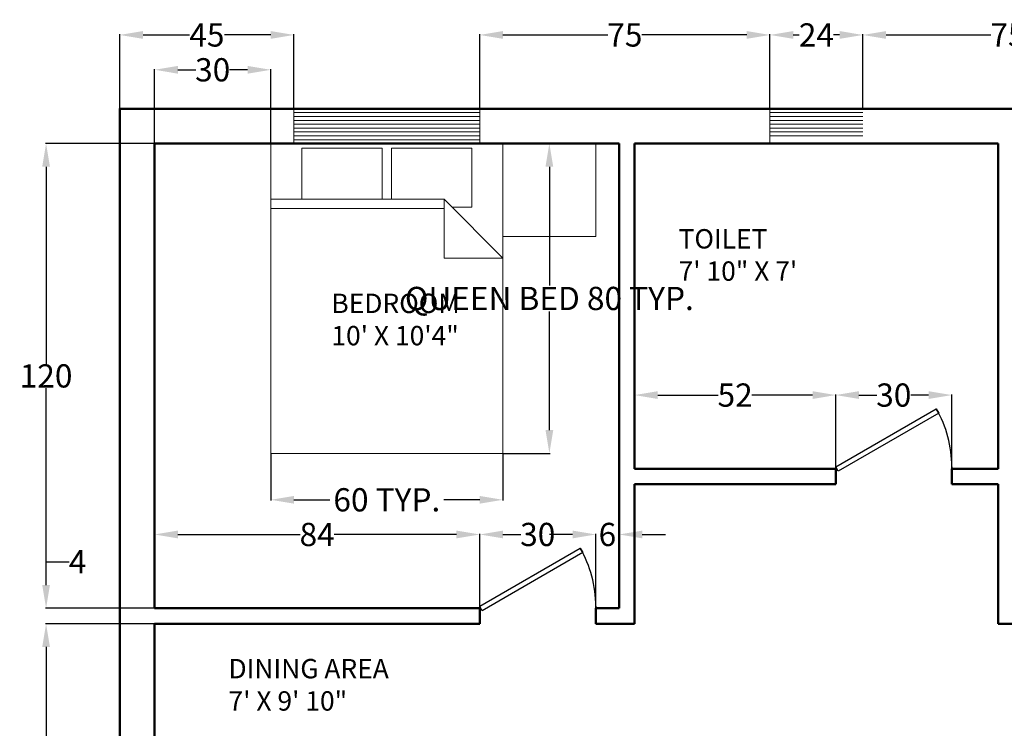
# Model space of a CAD drawing. Units: inches. Extents: x -8 to 445, y -363 to 43.
# Tile 2 of 3: x -8 to 246, y -140 to 43. Entities that reach past the tile are written whole.
import ezdxf

# ---------------------------------------------------------------- set-up
doc = ezdxf.new("R2010")
doc.units = ezdxf.units.IN
doc.header["$MEASUREMENT"] = 0
for name, color, linetype, lineweight in [('A-ANNO-DIMS', 2, 'Continuous', 18), ('A-AREA-IDEN', 7, 'Continuous', 18), ('A-FURN', 8, 'Continuous', 18), ('A-WALL', 7, 'Continuous', 50), ('DOORS', 43, 'Continuous', 25), ('WINDOWS', 140, 'Continuous', 18)]:
    doc.layers.add(name, color=color, linetype=linetype, lineweight=lineweight)
doc.styles.get("Standard").update_dxf_attribs({"font": 'arial.ttf'})
doc.dimstyles.get("Standard").update_dxf_attribs({"dimtxt": 6, "dimasz": 6, "dimexe": 0.18, "dimexo": 0.0625, "dimgap": 0.09, "dimtad": 0, "dimtih": 1, "dimtoh": 1, "dimdec": 0, "dimzin": 0, "dimdsep": 46, "dimlunit": 4, "dimtxsty": 'Standard', "dimcen": 0.09, "dimadec": 0, "dimazin": 0, "dimtfac": 1, "dimtdec": 0, "dimtofl": 0, "dimtmove": 0, "dimatfit": 3, "dimfxl": 1, "dimtolj": 1, "dimtzin": 0, "dimarcsym": 0})

# ---------------------------------------------------------------- blocks, each defined once
blk = doc.blocks.new('*U2')
for p, q in [((0, 0), (0, -6)), ((40, 0), (40, -6))]:
    blk.add_line(p, q)
blk.add_lwpolyline([(0, 0), (34.64, 20), (35.52, 18.48), (0.87, -1.52)], close=True)
blk.add_arc((0, 0), 40, 0, 30)
blk = doc.blocks.new('Bed - Queen')
for p, q in [((0, -80.00003), (0, 0)), ((0, 0), (59.99999, 0)), ((59.99999, 0), (59.99999, -80.00003)), ((7.99999, -1.2), (28.79998, -1.2)), ((7.99999, -14.4), (7.99999, -1.2)), ((28.79998, -1.2), (28.79998, -14.4)), ((31.19999, -1.2), (51.99999, -1.2)), ((31.19999, -14.4), (31.19999, -1.2)), ((51.99999, -1.2), (51.99999, -16.4)), ((0, -14.4), (44.8, -14.4)), ((59.99999, -29.6), (44.8, -14.4)), ((44.8, -14.4), (44.8, -29.6)), ((44.8, -16.8), (0, -16.8)), ((51.99999, -16.4), (46.79936, -16.4)), ((44.8, -29.6), (59.99999, -29.6)), ((59.99999, -80.00003), (0, -80.00003))]:
    blk.add_line(p, q)
blk = doc.blocks.new('WIN-48IN')
for p, q in [((0, 0), (0, 9)), ((0, 9), (48, 9)), ((0, 8), (48, 8)), ((48, 9), (48, 0)), ((0, 7), (48, 7)), ((0, 6), (48, 6)), ((0, 5), (48, 5)), ((0, 4), (48, 4)), ((0, 3), (48, 3)), ((0, 2), (48, 2)), ((48, 1), (0, 1)), ((48, 0), (0, 0))]:
    blk.add_line(p, q)
blk = doc.blocks.new('NIGHTSTAND-24IN')
blk.add_lwpolyline([(0, 24), (24, 24), (24, 0), (0, 0)], close=True)
blk = doc.blocks.new('*D17')
at = {"layer": 'A-ANNO-DIMS', "color": 0, "lineweight": -2, "transparency": 16777216}
for p, q in [((116.95, 10.91), (129.07, 10.91)), ((128.89, 4.91), (128.89, -25.71)), ((128.89, -63.09), (128.89, -32.47)), ((116.95, -69.09), (129.07, -69.09))]:
    blk.add_line(p, q, dxfattribs=at)
at = {"layer": 'A-ANNO-DIMS', "color": 0, "transparency": 16777216}
for points in [[(127.89, 4.91), (129.89, 4.91), (128.89, 10.91)], [(127.89, -63.09), (129.89, -63.09), (128.89, -69.09)]]:
    blk.add_solid(points, dxfattribs=at)
at = {"layer": 'Defpoints', "color": 0, "transparency": 16777216}
for p in [(116.89, 10.91), (128.89, 10.91), (116.89, -69.09)]:
    blk.add_point(p, dxfattribs=at)
at = {"layer": 'A-ANNO-DIMS', "color": 0, "transparency": 16777216, "insert": (128.89, -29.09), "char_height": 6, "attachment_point": 5}
blk.add_mtext('\\A1;QUEEN BED 80 TYP.', dxfattribs=at)
blk = doc.blocks.new('*D18')
at = {"layer": 'A-ANNO-DIMS', "color": 0, "lineweight": -2, "transparency": 16777216}
for p, q in [((56.89, -69.15), (56.89, -81.27)), ((116.89, -69.15), (116.89, -81.27)), ((62.89, -81.09), (72.18, -81.09)), ((110.89, -81.09), (101.6, -81.09))]:
    blk.add_line(p, q, dxfattribs=at)
at = {"layer": 'A-ANNO-DIMS', "color": 0, "transparency": 16777216}
for points in [[(62.89, -80.09), (62.89, -82.09), (56.89, -81.09)], [(110.89, -80.09), (110.89, -82.09), (116.89, -81.09)]]:
    blk.add_solid(points, dxfattribs=at)
at = {"layer": 'Defpoints', "color": 0, "transparency": 16777216}
for p in [(56.89, -69.09), (116.89, -69.09), (116.89, -81.09)]:
    blk.add_point(p, dxfattribs=at)
at = {"layer": 'A-ANNO-DIMS', "color": 0, "transparency": 16777216, "insert": (86.89, -81.09), "char_height": 6, "attachment_point": 5}
blk.add_mtext('\\A1;60 TYP.', dxfattribs=at)
blk = doc.blocks.new('*D35')
at = {"layer": 'A-ANNO-DIMS', "color": 0, "lineweight": -2, "transparency": 16777216}
for p, q in [((17.89, 19.97), (17.89, 39.14)), ((23.89, 38.96), (35.86, 38.96)), ((56.89, 38.96), (44.92, 38.96)), ((62.89, 19.97), (62.89, 39.14))]:
    blk.add_line(p, q, dxfattribs=at)
at = {"layer": 'A-ANNO-DIMS', "color": 0, "transparency": 16777216}
for points in [[(23.89, 39.96), (23.89, 37.96), (17.89, 38.96)], [(56.89, 39.96), (56.89, 37.96), (62.89, 38.96)]]:
    blk.add_solid(points, dxfattribs=at)
at = {"layer": 'Defpoints', "color": 0, "transparency": 16777216}
for p in [(62.89, 38.96), (17.89, 19.91), (62.89, 19.91)]:
    blk.add_point(p, dxfattribs=at)
at = {"layer": 'A-ANNO-DIMS', "color": 0, "transparency": 16777216, "insert": (40.39, 38.96), "char_height": 6, "attachment_point": 5}
blk.add_mtext('\\A1;45', dxfattribs=at)
blk = doc.blocks.new('*D36')
at = {"layer": 'A-ANNO-DIMS', "color": 0, "lineweight": -2, "transparency": 16777216}
for p, q in [((110.89, 19.97), (110.89, 39.14)), ((116.89, 38.96), (144, 38.96)), ((179.89, 38.96), (152.77, 38.96)), ((185.89, 19.97), (185.89, 39.14))]:
    blk.add_line(p, q, dxfattribs=at)
at = {"layer": 'A-ANNO-DIMS', "color": 0, "transparency": 16777216}
for points in [[(116.89, 39.96), (116.89, 37.96), (110.89, 38.96)], [(179.89, 39.96), (179.89, 37.96), (185.89, 38.96)]]:
    blk.add_solid(points, dxfattribs=at)
at = {"layer": 'Defpoints', "color": 0, "transparency": 16777216}
for p in [(185.89, 38.96), (110.89, 19.91), (185.89, 19.91)]:
    blk.add_point(p, dxfattribs=at)
at = {"layer": 'A-ANNO-DIMS', "color": 0, "transparency": 16777216, "insert": (148.39, 38.96), "char_height": 6, "attachment_point": 5}
blk.add_mtext('\\A1;75', dxfattribs=at)
blk = doc.blocks.new('*D37')
at = {"layer": 'A-ANNO-DIMS', "color": 0, "lineweight": -2, "transparency": 16777216}
for p, q in [((185.89, 19.97), (185.89, 39.14)), ((191.89, 38.96), (193.46, 38.96)), ((203.89, 38.96), (202.31, 38.96)), ((209.89, 19.97), (209.89, 39.14))]:
    blk.add_line(p, q, dxfattribs=at)
at = {"layer": 'A-ANNO-DIMS', "color": 0, "transparency": 16777216}
for points in [[(191.89, 39.96), (191.89, 37.96), (185.89, 38.96)], [(203.89, 39.96), (203.89, 37.96), (209.89, 38.96)]]:
    blk.add_solid(points, dxfattribs=at)
at = {"layer": 'Defpoints', "color": 0, "transparency": 16777216}
for p in [(209.89, 38.96), (185.89, 19.91), (209.89, 19.91)]:
    blk.add_point(p, dxfattribs=at)
at = {"layer": 'A-ANNO-DIMS', "color": 0, "transparency": 16777216, "insert": (197.89, 38.96), "char_height": 6, "attachment_point": 5}
blk.add_mtext('\\A1;24', dxfattribs=at)
blk = doc.blocks.new('*D38')
at = {"layer": 'A-ANNO-DIMS', "color": 0, "lineweight": -2, "transparency": 16777216}
for p, q in [((209.89, 19.97), (209.89, 39.14)), ((215.89, 38.96), (243, 38.96)), ((278.89, 38.96), (251.77, 38.96)), ((284.89, 19.97), (284.89, 39.14))]:
    blk.add_line(p, q, dxfattribs=at)
at = {"layer": 'A-ANNO-DIMS', "color": 0, "transparency": 16777216}
for points in [[(215.89, 39.96), (215.89, 37.96), (209.89, 38.96)], [(278.89, 39.96), (278.89, 37.96), (284.89, 38.96)]]:
    blk.add_solid(points, dxfattribs=at)
at = {"layer": 'Defpoints', "color": 0, "transparency": 16777216}
for p in [(284.89, 38.96), (209.89, 19.91), (284.89, 19.91)]:
    blk.add_point(p, dxfattribs=at)
at = {"layer": 'A-ANNO-DIMS', "color": 0, "transparency": 16777216, "insert": (247.39, 38.96), "char_height": 6, "attachment_point": 5}
blk.add_mtext('\\A1;75', dxfattribs=at)
blk = doc.blocks.new('*D39')
at = {"layer": 'A-ANNO-DIMS', "color": 0, "lineweight": -2, "transparency": 16777216}
for p, q in [((26.82, 10.91), (-1.34, 10.91)), ((-1.16, 4.91), (-1.16, -45.94)), ((-1.16, -103.09), (-1.16, -52.24)), ((26.82, -109.09), (-1.34, -109.09))]:
    blk.add_line(p, q, dxfattribs=at)
at = {"layer": 'A-ANNO-DIMS', "color": 0, "transparency": 16777216}
for points in [[(-2.16, 4.91), (-0.16, 4.91), (-1.16, 10.91)], [(-2.16, -103.09), (-0.16, -103.09), (-1.16, -109.09)]]:
    blk.add_solid(points, dxfattribs=at)
at = {"layer": 'Defpoints', "color": 0, "transparency": 16777216}
for p in [(-1.16, 10.91), (26.89, 10.91), (26.89, -109.09)]:
    blk.add_point(p, dxfattribs=at)
at = {"layer": 'A-ANNO-DIMS', "color": 0, "transparency": 16777216, "insert": (-1.16, -49.09), "char_height": 6, "attachment_point": 5}
blk.add_mtext('\\A1;120', dxfattribs=at)
blk = doc.blocks.new('*D40')
at = {"layer": 'A-ANNO-DIMS', "color": 0, "lineweight": -2, "transparency": 16777216}
for p, q in [((-1.16, -103.09), (-1.16, -97.09)), ((-1.16, -97.09), (4.84, -97.09)), ((26.82, -109.09), (-1.34, -109.09)), ((26.82, -113.09), (-1.34, -113.09)), ((-1.16, -119.09), (-1.16, -125.09))]:
    blk.add_line(p, q, dxfattribs=at)
at = {"layer": 'A-ANNO-DIMS', "color": 0, "transparency": 16777216}
for points in [[(-2.16, -103.09), (-0.16, -103.09), (-1.16, -109.09)], [(-2.16, -119.09), (-0.16, -119.09), (-1.16, -113.09)]]:
    blk.add_solid(points, dxfattribs=at)
at = {"layer": 'Defpoints', "color": 0, "transparency": 16777216}
for p in [(-1.16, -109.09), (26.89, -109.09), (26.89, -113.09)]:
    blk.add_point(p, dxfattribs=at)
at = {"layer": 'A-ANNO-DIMS', "color": 0, "transparency": 16777216, "insert": (7, -97.09), "char_height": 6, "attachment_point": 5}
blk.add_mtext('\\A1;4', dxfattribs=at)
blk = doc.blocks.new('*D41')
at = {"layer": 'A-ANNO-DIMS', "color": 0, "lineweight": -2, "transparency": 16777216}
for p, q in [((26.82, -113.09), (-1.34, -113.09)), ((-1.16, -119.09), (-1.16, -168.94)), ((-1.16, -225.09), (-1.16, -175.24)), ((26.82, -231.09), (-1.34, -231.09))]:
    blk.add_line(p, q, dxfattribs=at)
at = {"layer": 'A-ANNO-DIMS', "color": 0, "transparency": 16777216}
for points in [[(-2.16, -119.09), (-0.16, -119.09), (-1.16, -113.09)], [(-2.16, -225.09), (-0.16, -225.09), (-1.16, -231.09)]]:
    blk.add_solid(points, dxfattribs=at)
at = {"layer": 'Defpoints', "color": 0, "transparency": 16777216}
for p in [(-1.16, -113.09), (26.89, -113.09), (26.89, -231.09)]:
    blk.add_point(p, dxfattribs=at)
at = {"layer": 'A-ANNO-DIMS', "color": 0, "transparency": 16777216, "insert": (-1.16, -172.09), "char_height": 6, "attachment_point": 5}
blk.add_mtext('\\A1;118', dxfattribs=at)
blk = doc.blocks.new('*D50')
at = {"layer": 'A-ANNO-DIMS', "color": 0, "lineweight": -2, "transparency": 16777216}
for p, q in [((110.89, -109.03), (110.89, -89.86)), ((116.89, -90.04), (121.51, -90.04)), ((134.89, -90.04), (130.26, -90.04)), ((140.89, -109.03), (140.89, -89.86))]:
    blk.add_line(p, q, dxfattribs=at)
at = {"layer": 'A-ANNO-DIMS', "color": 0, "transparency": 16777216}
for points in [[(116.89, -89.04), (116.89, -91.04), (110.89, -90.04)], [(134.89, -89.04), (134.89, -91.04), (140.89, -90.04)]]:
    blk.add_solid(points, dxfattribs=at)
at = {"layer": 'Defpoints', "color": 0, "transparency": 16777216}
for p in [(140.89, -90.04), (110.89, -109.09), (140.89, -109.09)]:
    blk.add_point(p, dxfattribs=at)
at = {"layer": 'A-ANNO-DIMS', "color": 0, "transparency": 16777216, "insert": (125.89, -90.04), "char_height": 6, "attachment_point": 5}
blk.add_mtext('\\A1;30', dxfattribs=at)
blk = doc.blocks.new('*D51')
at = {"layer": 'A-ANNO-DIMS', "color": 0, "lineweight": -2, "transparency": 16777216}
for p, q in [((26.89, -109.03), (26.89, -89.86)), ((32.89, -90.04), (64.51, -90.04)), ((104.89, -90.04), (73.27, -90.04)), ((110.89, -109.03), (110.89, -89.86))]:
    blk.add_line(p, q, dxfattribs=at)
at = {"layer": 'A-ANNO-DIMS', "color": 0, "transparency": 16777216}
for points in [[(32.89, -89.04), (32.89, -91.04), (26.89, -90.04)], [(104.89, -89.04), (104.89, -91.04), (110.89, -90.04)]]:
    blk.add_solid(points, dxfattribs=at)
at = {"layer": 'Defpoints', "color": 0, "transparency": 16777216}
for p in [(110.89, -90.04), (26.89, -109.09), (110.89, -109.09)]:
    blk.add_point(p, dxfattribs=at)
at = {"layer": 'A-ANNO-DIMS', "color": 0, "transparency": 16777216, "insert": (68.89, -90.04), "char_height": 6, "attachment_point": 5}
blk.add_mtext('\\A1;84', dxfattribs=at)
blk = doc.blocks.new('*D52')
at = {"layer": 'A-ANNO-DIMS', "color": 0, "lineweight": -2, "transparency": 16777216}
for p, q in [((134.887242, -90.040687), (128.887242, -90.040687)), ((140.887242, -109.028187), (140.887242, -89.860687)), ((146.887242, -109.028187), (146.887242, -89.860687)), ((152.887242, -90.040687), (158.887242, -90.040687))]:
    blk.add_line(p, q, dxfattribs=at)
at = {"layer": 'A-ANNO-DIMS', "color": 0, "transparency": 16777216}
for points in [[(134.887242, -89.040687), (134.887242, -91.040687), (140.887242, -90.040687)], [(152.887242, -89.040687), (152.887242, -91.040687), (146.887242, -90.040687)]]:
    blk.add_solid(points, dxfattribs=at)
at = {"layer": 'Defpoints', "color": 0, "transparency": 16777216}
for p in [(146.887242, -90.040687), (140.887242, -109.090687), (146.887242, -109.090687)]:
    blk.add_point(p, dxfattribs=at)
at = {"layer": 'A-ANNO-DIMS', "color": 0, "transparency": 16777216, "insert": (143.887242, -90.040687), "char_height": 6, "attachment_point": 5}
blk.add_mtext('\\A1;6', dxfattribs=at)
blk = doc.blocks.new('*D53')
at = {"layer": 'A-ANNO-DIMS', "color": 0, "lineweight": -2, "transparency": 16777216}
for p, q in [((150.89, -73.03), (150.89, -53.86)), ((156.89, -54.04), (172.53, -54.04)), ((196.89, -54.04), (181.24, -54.04)), ((202.89, -73.03), (202.89, -53.86))]:
    blk.add_line(p, q, dxfattribs=at)
at = {"layer": 'A-ANNO-DIMS', "color": 0, "transparency": 16777216}
for points in [[(156.89, -53.04), (156.89, -55.04), (150.89, -54.04)], [(196.89, -53.04), (196.89, -55.04), (202.89, -54.04)]]:
    blk.add_solid(points, dxfattribs=at)
at = {"layer": 'Defpoints', "color": 0, "transparency": 16777216}
for p in [(202.89, -54.04), (150.89, -73.09), (202.89, -73.09)]:
    blk.add_point(p, dxfattribs=at)
at = {"layer": 'A-ANNO-DIMS', "color": 0, "transparency": 16777216, "insert": (176.89, -54.04), "char_height": 6, "attachment_point": 5}
blk.add_mtext('\\A1;52', dxfattribs=at)
blk = doc.blocks.new('*D54')
at = {"layer": 'A-ANNO-DIMS', "color": 0, "lineweight": -2, "transparency": 16777216}
for p, q in [((202.89, -73.03), (202.89, -53.86)), ((208.89, -54.04), (213.51, -54.04)), ((226.89, -54.04), (222.26, -54.04)), ((232.89, -73.03), (232.89, -53.86))]:
    blk.add_line(p, q, dxfattribs=at)
at = {"layer": 'A-ANNO-DIMS', "color": 0, "transparency": 16777216}
for points in [[(208.89, -53.04), (208.89, -55.04), (202.89, -54.04)], [(226.89, -53.04), (226.89, -55.04), (232.89, -54.04)]]:
    blk.add_solid(points, dxfattribs=at)
at = {"layer": 'Defpoints', "color": 0, "transparency": 16777216}
for p in [(232.89, -54.04), (202.89, -73.09), (232.89, -73.09)]:
    blk.add_point(p, dxfattribs=at)
at = {"layer": 'A-ANNO-DIMS', "color": 0, "transparency": 16777216, "insert": (217.89, -54.04), "char_height": 6, "attachment_point": 5}
blk.add_mtext('\\A1;30', dxfattribs=at)
blk = doc.blocks.new('*D61')
at = {"layer": 'A-ANNO-DIMS', "color": 0, "lineweight": -2, "transparency": 16777216}
for p, q in [((26.89, 10.97), (26.89, 30.14)), ((32.89, 29.96), (37.51, 29.96)), ((50.89, 29.96), (46.26, 29.96)), ((56.89, 10.97), (56.89, 30.14))]:
    blk.add_line(p, q, dxfattribs=at)
at = {"layer": 'A-ANNO-DIMS', "color": 0, "transparency": 16777216}
for points in [[(32.89, 30.96), (32.89, 28.96), (26.89, 29.96)], [(50.89, 30.96), (50.89, 28.96), (56.89, 29.96)]]:
    blk.add_solid(points, dxfattribs=at)
at = {"layer": 'Defpoints', "color": 0, "transparency": 16777216}
for p in [(56.89, 29.96), (26.89, 10.91), (56.89, 10.91)]:
    blk.add_point(p, dxfattribs=at)
at = {"layer": 'A-ANNO-DIMS', "color": 0, "transparency": 16777216, "insert": (41.89, 29.96), "char_height": 6, "attachment_point": 5}
blk.add_mtext('\\A1;30', dxfattribs=at)

msp = doc.modelspace()

# ---------------------------------------------------------------- linework, layer by layer
at = {"layer": 'A-WALL'}
for p, q in [((26.8872, 10.9093), (146.8872, 10.9093)), ((26.8872, -109.0907), (26.8872, 10.9093)), ((146.8872, -109.0907), (146.8872, 10.9093)), ((150.8872, -73.0907), (150.8872, 10.9093)), ((150.8872, 10.9093), (244.8872, 10.9093)), ((244.8872, 10.9093), (244.8872, -73.0907)), ((150.8872, -73.0907), (202.8872, -73.0907)), ((202.8872, -73.0907), (202.8872, -77.0907)), ((232.8872, -73.0907), (232.8872, -77.0907)), ((232.8872, -73.0907), (244.8872, -73.0907)), ((150.8872, -113.0907), (150.8872, -77.0907)), ((150.8872, -77.0907), (202.8872, -77.0907)), ((232.8872, -77.0907), (244.8872, -77.0907)), ((244.8872, -77.0907), (244.8872, -113.0907)), ((26.8872, -109.0907), (110.8872, -109.0907)), ((110.8872, -109.0907), (110.8872, -113.0907)), ((140.8872, -109.0907), (140.8872, -113.0907)), ((140.8872, -109.0907), (146.8872, -109.0907)), ((26.8872, -113.0907), (110.8872, -113.0907)), ((26.8872, -231.0907), (26.8872, -113.0907)), ((140.8872, -113.0907), (150.8872, -113.0907)), ((244.8872, -113.0907), (254.8872, -113.0907))]:
    msp.add_line(p, q, dxfattribs=at)
msp.add_lwpolyline([(182.8872, -340.0907), (17.8872, -340.0907), (17.8872, 19.9093), (377.8872, 19.9093), (377.8872, -340.0907), (212.8872, -340.0907)], dxfattribs=at)
at = {"layer": 'WINDOWS'}
for p, q in [((209.8872, 19.9093), (185.8872, 19.9093)), ((185.8872, 19.9093), (185.8872, 10.9093)), ((185.8872, 18.9093), (209.8872, 18.9093)), ((185.8872, 17.9093), (209.8872, 17.9093)), ((185.8872, 16.9093), (209.8872, 16.9093)), ((185.8872, 15.9093), (209.8872, 15.9093)), ((185.8872, 14.9093), (209.8872, 14.9093)), ((185.8872, 13.9093), (209.8872, 13.9093)), ((185.8872, 12.9093), (209.8872, 12.9093))]:
    msp.add_line(p, q, dxfattribs=at)

# ---------------------------------------------------------------- block references
at = {"layer": 'A-FURN'}
for name, p in [('Bed - Queen', (56.8872, 10.9093)), ('NIGHTSTAND-24IN', (116.887, -13.091))]:
    msp.add_blockref(name, p, dxfattribs=at)
at = {"layer": 'DOORS', "xscale": 0.75, "yscale": 0.75, "zscale": 0.75}
for p in [(202.8872, -72.5907), (110.8872, -108.5907)]:
    msp.add_blockref('*U2', p, dxfattribs=at)
at = {"layer": 'WINDOWS'}
msp.add_blockref('WIN-48IN', (62.887, 10.909), dxfattribs=at)

# ---------------------------------------------------------------- texts
at = {"layer": 'A-AREA-IDEN', "char_height": 5, "attachment_point": 1}
for s, width, insert in [('TOILET \\P7\' 10" X 7\'', 70.512809, (162.2804, -11.1894)), ('BEDROOM \\P10\' X 10\'4"', 84.445494, (72.5661, -27.8547)), ('DINING AREA \\P7\' X 9\' 10"', 79.030752, (45.973, -122.192))]:
    msp.add_mtext_dynamic_manual_height_columns(s, width=width, gutter_width=1, heights=[0], dxfattribs=dict(at, insert=insert))

# ---------------------------------------------------------------- dimensions: what is measured, and where the dimension line sits
at = {"layer": 'A-ANNO-DIMS'}
for base, p1, p2, picture, middle in [((62.8872, 38.9593), (17.8872, 19.9093), (62.8872, 19.9093), '*D35', (40.3872, 38.9593)), ((185.8872, 38.9593), (110.8872, 19.9093), (185.8872, 19.9093), '*D36', (148.3872, 38.9593)), ((209.8872, 38.9593), (185.8872, 19.9093), (209.8872, 19.9093), '*D37', (197.8872, 38.9593)), ((284.8872, 38.9593), (209.8872, 19.9093), (284.8872, 19.9093), '*D38', (247.3872, 38.9593)), ((202.8872, -54.0407), (150.8872, -73.0907), (202.8872, -73.0907), '*D53', (176.8872, -54.0407)), ((110.8872, -90.0407), (26.8872, -109.0907), (110.8872, -109.0907), '*D51', (68.8872, -90.0407)), ((140.8872, -90.0407), (110.8872, -109.0907), (140.8872, -109.0907), '*D50', (125.8872, -90.0407)), ((146.8872, -90.0407), (140.8872, -109.0907), (146.8872, -109.0907), '*D52', (143.8872, -90.0407))]:
    dim = msp.add_linear_dim(base=base, p1=p1, p2=p2, dimstyle='Standard', override={"dimdec": 0, "dimlfac": 1, "dimrnd": 0, "dimzin": 0, "dimdsep": 46, "dimlunit": 2}, dxfattribs=at)
    dim.commit()
    dim.dimension.update_dxf_attribs({"geometry": picture, "text_midpoint": middle})
for base, p1, p2, angle, picture, middle in [((56.8872, 29.9593), (26.8872, 10.9093), (56.8872, 10.9093), 0, '*D61', (41.8872, 29.9593)), ((-1.1628, 10.9093), (26.8872, -109.0907), (26.8872, 10.9093), 90, '*D39', (-1.1628, -49.0907)), ((232.8872, -54.0407), (202.8872, -73.0907), (232.8872, -73.0907), 0, '*D54', (217.8872, -54.0407)), ((-1.1628, -109.0907), (26.8872, -113.0907), (26.8872, -109.0907), 90, '*D40', (7.0023, -97.0907)), ((-1.1628, -113.0907), (26.8872, -231.0907), (26.8872, -113.0907), 90, '*D41', (-1.1628, -172.0907))]:
    dim = msp.add_linear_dim(base=base, p1=p1, p2=p2, angle=angle, dimstyle='Standard', override={"dimdec": 0, "dimlfac": 1, "dimrnd": 0, "dimzin": 0, "dimdsep": 46, "dimlunit": 2}, dxfattribs=at)
    dim.commit()
    dim.dimension.update_dxf_attribs({"geometry": picture, "text_midpoint": middle})
dim = msp.add_linear_dim(base=(128.8872, 10.9093), p1=(116.8872, -69.0907), p2=(116.8872, 10.9093), angle=90, text='QUEEN BED <> TYP.', dimstyle='Standard', override={"dimdec": 0, "dimlfac": 1, "dimrnd": 0, "dimzin": 0, "dimdsep": 46, "dimlunit": 2}, dxfattribs=at)
dim.commit()
dim.dimension.update_dxf_attribs({"geometry": '*D17', "text_midpoint": (128.8872, -29.0907)})
dim = msp.add_linear_dim(base=(116.8872, -81.0907), p1=(56.8872, -69.0907), p2=(116.8872, -69.0907), text='<> TYP.', dimstyle='Standard', override={"dimdec": 0, "dimlfac": 1, "dimrnd": 0, "dimzin": 0, "dimdsep": 46, "dimlunit": 2}, dxfattribs=at)
dim.commit()
dim.dimension.update_dxf_attribs({"geometry": '*D18', "text_midpoint": (86.8872, -81.0907)})

doc.saveas('drawing.dxf')
